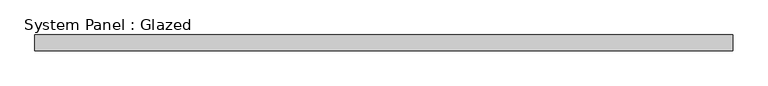
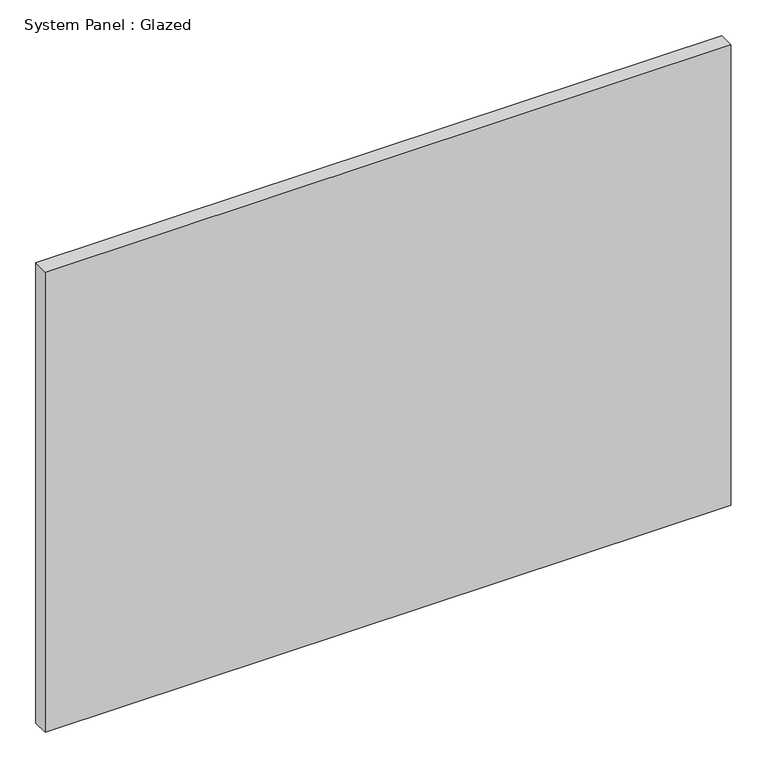
"""IFC4 building model written with IfcOpenShell, lengths in millimetres: plate geometry, System Panel : Glazed."""

from ifc_helpers import new_model, si_unit, origin, origin_with_axes, place, context, project, spatial, polyline, outline, extrude, source, transform, mapped, element, save


def system_panel_glazed_4864a337(model_context):
    return source(origin(), model_context, "Body", "SweptSolid", [
        extrude(outline(polyline([(551.392122, 19.05), (-551.392122, 19.05), (-551.392122, 44.45), (551.392122, 44.45), (551.392122, 19.05)])), origin_with_axes(), (0.0, 0.0, 1.0), 782.3541168),
    ])


if __name__ == "__main__":
    model = new_model("IFC4")
    model_context = context("Model", 3, world=origin())
    ifc_project = project(units=[si_unit("LENGTHUNIT", "METRE", prefix="MILLI")], contexts=[model_context])
    site = spatial("IfcSite", under=ifc_project)
    building = spatial("IfcBuilding", under=site)
    placement = place(None, origin())
    system_panel_glazed_shape = system_panel_glazed_4864a337(model_context)
    element("IfcPlate", 1, ObjectType="System Panel : Glazed", at=placement, inside=building, context=model_context, shape_type="MappedRepresentation", body=[
        mapped(system_panel_glazed_shape, transform((0.0, 0.0, 0.0), x_axis=(1.0, 0.0, 0.0), y_axis=(0.0, 1.0, 0.0), z_axis=(0.0, 0.0, 1.0))),
    ])
    save(model, "model.ifc")

# Revit data of these elements
# Type "System Panel : Glazed"
#   Construction Type Id = "GSP4R"
#   Analytic Construction = "1/8 in Pilkington single glazing"
#   Visual Light Transmittance = 0.9
#   Solar Heat Gain Coefficient = 0.86
#   Heat Transfer Coefficient (U) = 1.18115 BTU/(h·ft²·°F)
# Element 1 (IfcPlate, "System Panel : Glazed")
#   Materials on its faces: "Glass"
# Materials
#   "Glass": class "Glass", colour RGB 0 128 192, transparency 0.75, Description = "Soda Lime Glass", Cost = 0
